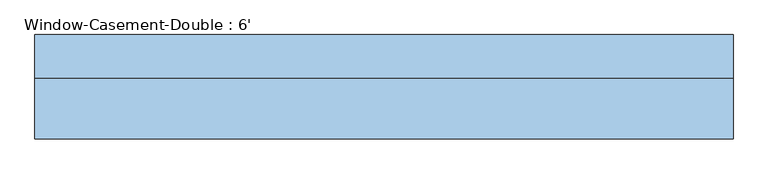
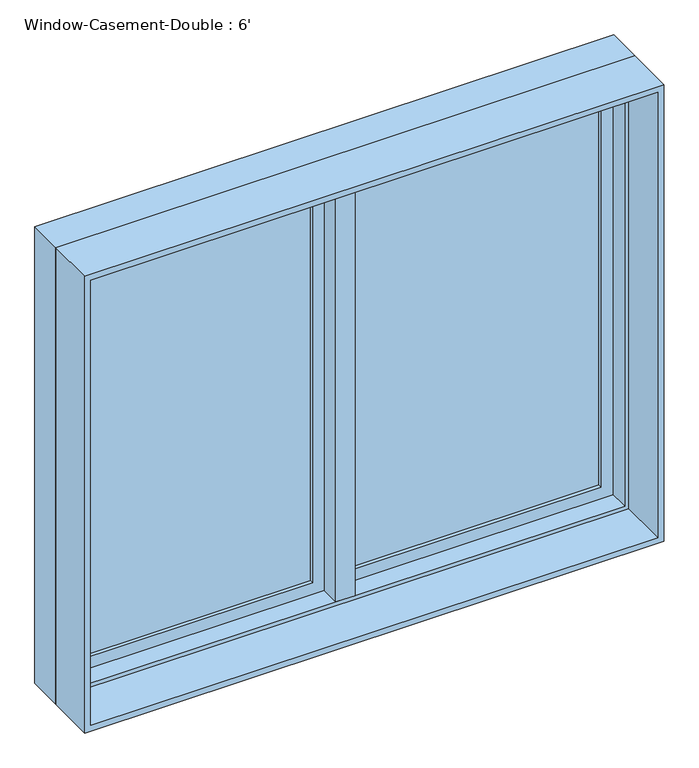
"""IFC4 building model written with IfcOpenShell, lengths in millimetres: window geometry, Window-Casement-Double : 6'."""

from ifc_helpers import new_model, si_unit, frame, origin, place, context, project, spatial, polyline, outline, extrude, faceted_brep, source, transform, mapped, element, save


def window_casement_double_6_75db422f(model_context):
    return source(origin(), model_context, "Body", "SolidModel", [
        faceted_brep([(9.525, 146.05, 2425.7), (-9.525, 146.05, 2425.7), (-9.525, 95.25, 2425.7), (9.525, 95.25, 2425.7), (9.525, 146.05, 927.1), (9.525, 95.25, 927.1), (-9.525, 95.25, 927.1), (-9.525, 146.05, 927.1), (-9.525, 95.25, 946.15), (-9.525, 95.25, 2406.65), (-30.1625, 95.25, 946.15), (-30.1625, 95.25, 2406.65), (-30.1625, 31.75, 946.15), (-30.1625, 31.75, 2406.65), (30.1625, 31.75, 946.15), (30.1625, 31.75, 2406.65), (30.1625, 95.25, 946.15), (30.1625, 95.25, 2406.65), (9.525, 95.25, 946.15), (9.525, 95.25, 2406.65)], [[[0, 1, 2, 3]], [[4, 5, 6, 7]], [[1, 0, 4, 7]], [[2, 1, 7, 6, 8, 9]], [[9, 8, 10, 11]], [[11, 10, 12, 13]], [[13, 12, 14, 15]], [[15, 14, 16, 17]], [[17, 16, 18, 19]], [[0, 3, 19, 18, 5, 4]], [[18, 8, 6, 5]], [[9, 19, 3, 2]], [[8, 18, 16, 14, 12, 10]], [[19, 9, 11, 13, 15, 17]]]),
        extrude(outline(polyline([(-66.675, 127.0), (-66.675, 120.65), (-844.55, 120.65), (-844.55, 127.0), (-66.675, 127.0)])), frame((0.0, 0.0, 984.25), z_axis=(0.0, 0.0, 1.0), x_axis=(1.0, 0.0, 0.0)), (0.0, 0.0, 1.0), 1384.3),
        extrude(outline(polyline([(-844.55, 107.95), (-844.55, 114.3), (-66.675, 114.3), (-66.675, 107.95), (-844.55, 107.95)])), frame((0.0, 0.0, 984.25), z_axis=(0.0, 0.0, 1.0), x_axis=(1.0, 0.0, 0.0)), (0.0, 0.0, 1.0), 1384.3),
        extrude(outline(polyline([(844.55, 127.0), (844.55, 120.65), (66.675, 120.65), (66.675, 127.0), (844.55, 127.0)])), frame((0.0, 0.0, 984.25), z_axis=(0.0, 0.0, 1.0), x_axis=(1.0, 0.0, 0.0)), (0.0, 0.0, 1.0), 1384.3),
        extrude(outline(polyline([(66.675, 107.95), (66.675, 114.3), (844.55, 114.3), (844.55, 107.95), (66.675, 107.95)])), frame((0.0, 0.0, 984.25), z_axis=(0.0, 0.0, 1.0), x_axis=(1.0, 0.0, 0.0)), (0.0, 0.0, 1.0), 1384.3),
        extrude(outline(polyline([(2425.7, -901.7), (927.1, -901.7), (927.1, -9.525), (2425.7, -9.525), (2425.7, -901.7)]), holes=[polyline([(2368.55, -66.675), (984.25, -66.675), (984.25, -844.55), (2368.55, -844.55), (2368.55, -66.675)])]), frame((0.0, 95.25, 0.0), z_axis=(0.0, 1.0, 0.0), x_axis=(0.0, 0.0, 1.0)), (0.0, 0.0, 1.0), 44.45),
        extrude(outline(polyline([(927.1, 901.7), (2425.7, 901.7), (2425.7, 9.525), (927.1, 9.525), (927.1, 901.7)]), holes=[polyline([(984.25, 66.675), (2368.55, 66.675), (2368.55, 844.55), (984.25, 844.55), (984.25, 66.675)])]), frame((0.0, 95.25, 0.0), z_axis=(0.0, 1.0, 0.0), x_axis=(0.0, 0.0, 1.0)), (0.0, 0.0, 1.0), 44.45),
        extrude(outline(polyline([(2438.4, -914.4), (914.4, -914.4), (914.4, 914.4), (2438.4, 914.4), (2438.4, -914.4)]), holes=[polyline([(2419.35, 895.35), (933.45, 895.35), (933.45, -895.35), (2419.35, -895.35), (2419.35, 895.35)])]), frame((0.0, -127.0, 0.0), z_axis=(0.0, 1.0, 0.0), x_axis=(0.0, 0.0, 1.0)), (0.0, 0.0, 1.0), 158.75),
        faceted_brep([(882.65, 95.25, 2406.65), (882.65, 31.75, 2406.65), (-882.65, 31.75, 2406.65), (-882.65, 95.25, 2406.65), (901.7, 146.05, 2425.7), (901.7, 95.25, 2425.7), (-901.7, 95.25, 2425.7), (-901.7, 146.05, 2425.7), (914.4, 31.75, 2438.4), (914.4, 146.05, 2438.4), (-914.4, 146.05, 2438.4), (-914.4, 31.75, 2438.4), (-882.65, 31.75, 946.15), (-882.65, 95.25, 946.15), (-901.7, 95.25, 927.1), (-901.7, 146.05, 927.1), (-914.4, 146.05, 914.4), (-914.4, 31.75, 914.4), (882.65, 31.75, 946.15), (882.65, 95.25, 946.15), (901.7, 95.25, 927.1), (901.7, 146.05, 927.1), (914.4, 146.05, 914.4), (914.4, 31.75, 914.4)], [[[0, 1, 2, 3]], [[4, 5, 6, 7]], [[8, 9, 10, 11]], [[3, 2, 12, 13]], [[7, 6, 14, 15]], [[11, 10, 16, 17]], [[13, 12, 18, 19]], [[15, 14, 20, 21]], [[17, 16, 22, 23]], [[11, 17, 23, 8], [1, 18, 12, 2]], [[19, 18, 1, 0]], [[5, 20, 14, 6], [3, 13, 19, 0]], [[21, 20, 5, 4]], [[23, 22, 9, 8]], [[9, 22, 16, 10], [7, 15, 21, 4]]]),
    ])


if __name__ == "__main__":
    model = new_model("IFC4")
    model_context = context("Model", 3, world=origin())
    ifc_project = project(units=[si_unit("LENGTHUNIT", "METRE", prefix="MILLI")], contexts=[model_context])
    site = spatial("IfcSite", under=ifc_project)
    building = spatial("IfcBuilding", under=site)
    placement = place(None, origin())
    window_casement_double_6_shape = window_casement_double_6_75db422f(model_context)
    element("IfcWindow", 1, ObjectType="Window-Casement-Double : 6'", at=placement, inside=building, context=model_context, shape_type="MappedRepresentation", body=[
        mapped(window_casement_double_6_shape, transform((0.0, 0.0, 0.0), x_axis=(1.0, 0.0, 0.0), y_axis=(0.0, 1.0, 0.0), z_axis=(0.0, 0.0, 1.0))),
    ])
    save(model, "model.ifc")

# Revit data of these elements
# Type "Window-Casement-Double : 6'"
#   Type Mark = "18"
#   Fire Rating = "0.5h"
#   Assembly Code = "B2020100"
#   Analytic Construction = "Double glazing - domestic"
#   Frame Extension [instance default] = 0' - 0 1/4"
#   Window Inset [instance default] = 0' - 0"
#   Wall Thickness [instance default] = 0' - 6"
#   Interior Wall Closure [instance default] = 0' - 2 1/4"
#   Half Width = 3' - 0"
#   Visual Light Transmittance = 0.81
#   Thermal Resistance (R) = 1.8146 (h·ft²·°F)/BTU
#   Solar Heat Gain Coefficient = 0.76
#   Rough Width = 6' - 0 1/2"
#   Rough Height = 5' - 0 1/2"
#   Height = 5' - 0"
#   Heat Transfer Coefficient (U) = 0.5511 BTU/(h·ft²·°F)
#   Exterior Wall Closure [instance default] = 0' - 1 1/4"
#   Extension Jamb [instance default] = 0' - 2 1/4"
#   Default Sill Height = 3' - 0"
#   Width = 6' - 0"
#   Muntin Visibility = yes
#   Interior Trim Visibility [instance default] = yes
#   Exterior Trim Visibility [instance default] = yes
#   Extension Jamb Visibility [instance default] = yes
#   Interior Trim Material = Wood - Stained
#   Muntin Pattern = Muntin Pattern_2x2 : Muntin Pattern_2x2
#   Interior Trim = Trim-Window-Interior-Flat : Picture Frame
#   Interior Frame Material = Wood - Stained
#   Glass Panel Material = Glass
#   Exterior Trim Material = Clad - White
#   Exterior Trim = Trim-Window-Exterior-Flat : with Sill
#   Exterior Frame Material = Clad - White
#   Wall Closure = (empty or 0)
# Element 1 (IfcWindow, "Window-Casement-Double : 6'")
#   Wall Thickness = 0' - 10"
#   Extension Jamb = 0' - 6 1/4"
#   Materials on its faces: "Wood - Stained", "Glass", "Clad - White"
# Materials
#   "Wood - Stained": class "Wood", colour RGB 224 178 126, transparency 0, Cost = 0
#   "Glass": class "Glass", colour RGB 0 128 192, transparency 0.75, Description = "Soda Lime Glass", Cost = 0
#   "Clad - White": class "Wood", colour RGB 242 242 238, transparency 0, Cost = 0
